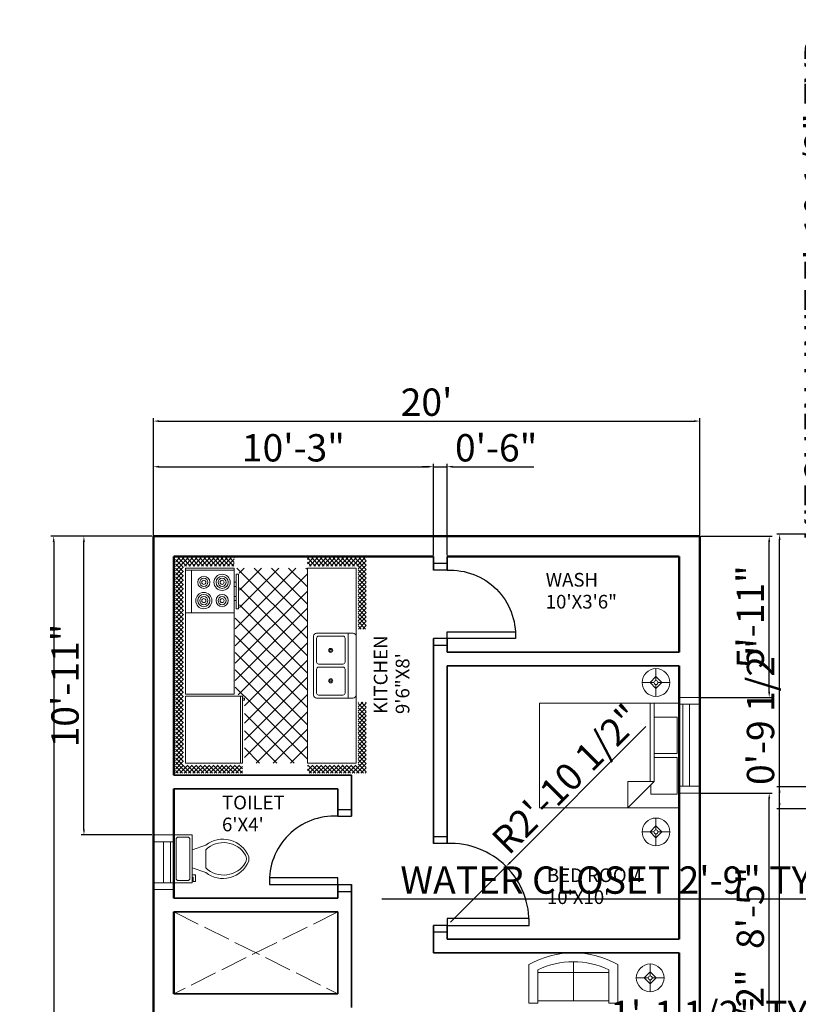
# Model space of a CAD drawing. Units: inches. Extents: x 2296 to 3335, y 495 to 1294.
# Tile 3 of 7: x 2296 to 2638, y 862 to 1294. Entities that reach past the tile are written whole.
import ezdxf

# ---------------------------------------------------------------- set-up
doc = ezdxf.new("R2010")
doc.units = ezdxf.units.IN
doc.linetypes.add('ACAD_ISO02W100', pattern=[15, 12, -3])
for name, color, linetype, lineweight in [('A-ANNO-DIMS', 2, 'Continuous', 18), ('A-AREA-IDEN', 7, 'Continuous', 18), ('A-FLOR-FIXT', 8, 'Continuous', 18), ('A-FLOR-OPEN', 7, 'ACAD_ISO02W100', 18), ('DOORS', 1, 'Continuous', 25), ('E-LITE', 2, 'Continuous', 18), ('FURNITURE', 2, 'Continuous', 18), ('INNER WALL', 6, 'Continuous', 35), ('OUTER WALL', 5, 'Continuous', 50), ('P-FIXT', 4, 'Continuous', 18), ('VENTILATOR', 4, 'Continuous', 18), ('WINDOWS', 3, 'Continuous', 18)]:
    doc.layers.add(name, color=color, linetype=linetype, lineweight=lineweight)
doc.styles.get("Standard").update_dxf_attribs({"font": 'arial.ttf'})
doc.dimstyles.new('ISO-25', dxfattribs={"dimtxt": 12, "dimasz": 2.5, "dimexe": 1.25, "dimexo": 0.625, "dimtad": 1, "dimdec": 1, "dimlunit": 3, "dimtxsty": 'Standard', "dimcen": 2.5, "dimadec": 0, "dimazin": 0, "dimtfac": 1, "dimtdec": 1, "dimtmove": 0, "dimatfit": 3, "dimfxl": 1, "dimarcsym": 0})

# ---------------------------------------------------------------- blocks, each defined once
blk = doc.blocks.new('Sofa - Roundback Loveseat 5 ft.')
for p, q in [((0, -32.44198), (0, -5.99998)), ((-24, -33.99998), (-24, -11.46958)), ((24.00004, -33.99998), (24.00004, -11.46958)), ((-23.9998, -13.38178), (23.99986, -13.38178)), ((-24, -32.44198), (24.00004, -32.44198))]:
    blk.add_line(p, q)
for points in [[(-24, -33.99998), (-30, -33.99998), (-30, -7.99998)], [(30.00004, -7.99998), (30.00004, -33.99998), (24.00004, -33.99998)]]:
    blk.add_lwpolyline(points)
for centre, radius, start, end in [((0, -60.24998), 60.24998, 60.13715, 119.8628), ((0, -61.38438), 55.38444, 64.32083, 115.6792)]:
    blk.add_arc(centre, radius, start, end)
blk = doc.blocks.new('Bed - Queen')
for p, q in [((0, -80.00003), (0, 0)), ((0, 0), (59.99999, 0)), ((59.99999, 0), (59.99999, -80.00003)), ((7.99999, -1.2), (28.79998, -1.2)), ((7.99999, -14.4), (7.99999, -1.2)), ((28.79998, -1.2), (28.79998, -14.4)), ((31.19999, -1.2), (51.99999, -1.2)), ((31.19999, -14.4), (31.19999, -1.2)), ((51.99999, -1.2), (51.99999, -16.4)), ((0, -14.4), (44.8, -14.4)), ((44.8, -16.8), (0, -16.8)), ((59.99999, -29.6), (44.8, -14.4)), ((44.8, -14.4), (44.8, -29.6)), ((51.99999, -16.4), (46.79936, -16.4)), ((44.8, -29.6), (59.99999, -29.6)), ((59.99999, -80.00003), (0, -80.00003))]:
    blk.add_line(p, q)
blk = doc.blocks.new('Kitchen Layout - 7 x 8 ft')
for p, q in [((-5, 81.32), (2.68, 89)), ((-5, 83.44), (0.56, 89)), ((-5, 85.56), (-1.56, 89)), ((-5, 87.68), (-3.68, 89)), ((-1, 84.97), (-5, 88.97)), ((1.09, 85), (-2.91, 89)), ((3.21, 85), (-0.79, 89)), ((0.81, 85), (4.81, 89)), ((5.34, 85), (1.34, 89)), ((2.93, 85), (6.93, 89)), ((7.46, 85), (3.46, 89)), ((5.05, 85), (9.05, 89)), ((9.58, 85), (5.58, 89)), ((7.17, 85), (11.17, 89)), ((11.7, 85), (7.7, 89)), ((9.29, 85), (13.29, 89)), ((13.82, 85), (9.82, 89)), ((11.41, 85), (15.41, 89)), ((15.94, 85), (11.94, 89)), ((13.53, 85), (17.53, 89)), ((18.06, 85), (14.06, 89)), ((15.65, 85), (19.65, 89)), ((20.18, 85), (16.18, 89)), ((17.78, 85), (21.78, 89)), ((22.31, 85), (18.31, 89)), ((19.9, 85), (23.9, 89)), ((24.43, 85), (20.43, 89)), ((22.02, 85), (26.02, 89)), ((26.55, 85), (22.55, 89)), ((24.14, 85), (28.14, 89)), ((28.67, 85), (24.67, 89)), ((26.26, 85), (30.26, 89)), ((30.79, 85), (26.79, 89)), ((28.38, 85), (32.38, 89)), ((32.91, 85), (28.91, 89)), ((30.5, 85), (34.5, 89)), ((35.03, 85), (31.03, 89)), ((32.63, 85), (36.63, 89)), ((37.16, 85), (33.16, 89)), ((34.75, 85), (38.75, 89)), ((39.28, 85), (35.28, 89)), ((36.87, 85), (40.87, 89)), ((41.4, 85), (37.4, 89)), ((38.99, 85), (42.99, 89)), ((43.52, 85), (39.52, 89)), ((41.11, 85), (45.11, 89)), ((45.64, 85), (41.64, 89)), ((43.23, 85), (47.23, 89)), ((47.76, 85), (43.76, 89)), ((45.35, 85), (49.35, 89)), ((49.88, 85), (45.88, 89)), ((47.47, 85), (51.47, 89)), ((52, 85), (48, 89)), ((49.6, 85), (53.6, 89)), ((54.13, 85), (50.13, 89)), ((51.72, 85), (55.72, 89)), ((56.25, 85), (52.25, 89)), ((53.84, 85), (57.84, 89)), ((58.37, 85), (54.37, 89)), ((55.96, 85), (59.96, 89)), ((60.49, 85), (56.49, 89)), ((58.08, 85), (62.08, 89)), ((62.61, 85), (58.61, 89)), ((60.2, 85), (64.2, 89)), ((64.73, 85), (60.73, 89)), ((62.32, 85), (66.32, 89)), ((66.85, 85), (62.85, 89)), ((64.45, 85), (68.45, 89)), ((68.97, 85), (64.97, 89)), ((66.57, 85), (70.57, 89)), ((71.1, 85), (67.1, 89)), ((68.69, 85), (72.69, 89)), ((73.22, 85), (69.22, 89)), ((70.81, 85), (74.81, 89)), ((75.34, 85), (71.34, 89)), ((72.93, 85), (76.93, 89)), ((77.46, 85), (73.46, 89)), ((75.05, 85), (79.05, 89)), ((79.58, 85), (75.58, 89)), ((77.17, 85), (81.17, 89)), ((81.7, 85), (77.7, 89)), ((79.29, 85), (83.29, 89)), ((83.82, 85), (79.82, 89)), ((81.42, 85), (85.42, 89)), ((85.95, 85), (81.95, 89)), ((83.54, 85), (87.54, 89)), ((88.07, 85), (84.07, 89)), ((85.66, 85), (89.66, 89)), ((90.19, 85), (86.19, 89)), ((87.78, 85), (91.78, 89)), ((92.31, 85), (88.31, 89)), ((89.9, 85), (93.9, 89)), ((94.43, 85), (90.43, 89)), ((92.02, 85), (96.02, 89)), ((96.55, 85), (92.55, 89)), ((94.14, 85), (98.14, 89)), ((101, 82.67), (94.67, 89)), ((96.27, 85), (100.27, 89)), ((101, 84.79), (96.79, 89)), ((97, 83.61), (101, 87.61)), ((101, 86.92), (98.92, 89)), ((-1, 82.85), (-5, 86.85)), ((-1, 80.73), (-5, 84.73)), ((-5, 79.19), (-1, 83.19)), ((-1, 78.61), (-5, 82.61)), ((34, 84), (96, 84)), ((34, 60), (34, 84)), ((96, 84), (96, 60)), ((97, 81.49), (101, 85.49)), ((101, 80.55), (97, 84.55)), ((97, 79.37), (101, 83.37)), ((101, 78.43), (97, 82.43)), ((-5, 77.07), (-1, 81.07)), ((-1, 76.49), (-5, 80.49)), ((-5, 74.95), (-1, 78.95)), ((-1, 74.36), (-5, 78.36)), ((74, 81), (95, 81)), ((97, 77.25), (101, 81.25)), ((101, 76.31), (97, 80.31)), ((97, 75.13), (101, 79.13)), ((101, 74.19), (97, 78.19)), ((-5, 72.83), (-1, 76.83)), ((-1, 72.24), (-5, 76.24)), ((-5, 70.71), (-1, 74.71)), ((-1, 70.12), (-5, 74.12)), ((97, 73.01), (101, 77.01)), ((101, 72.07), (97, 76.07)), ((97, 70.89), (101, 74.89)), ((101, 69.95), (97, 73.95)), ((97, 68.76), (101, 72.76)), ((-5, 68.59), (-1, 72.59)), ((-1, 68), (-5, 72)), ((-5, 66.47), (-1, 70.47)), ((-1, 65.88), (-5, 69.88)), ((-5, 64.35), (-1, 68.35)), ((101, 67.82), (97, 71.82)), ((97, 66.64), (101, 70.64)), ((101, 65.7), (97, 69.7)), ((97, 64.52), (101, 68.52)), ((-1, 63.76), (-5, 67.76)), ((-5, 62.22), (-1, 66.22)), ((-1, 61.64), (-5, 65.64)), ((-5, 60.1), (-1, 64.1)), ((-1, 59.52), (-5, 63.52)), ((101, 63.58), (97, 67.58)), ((97, 62.4), (101, 66.4)), ((101, 61.46), (97, 65.46)), ((97, 60.28), (101, 64.28)), ((100.34, 60), (97, 63.34)), ((-5, 57.98), (-1, 61.98)), ((-1, 57.39), (-5, 61.39)), ((-1.73, 56), (-5, 59.27)), ((-4.86, 56), (-1, 59.86)), ((10.4, 24), (45.9, 59.5)), ((18.88, 24), (54.38, 59.5)), ((27.37, 24), (62.87, 59.5)), ((33.03, 55.11), (37.41, 59.5)), ((96, 60), (34, 60)), ((35.85, 24), (71.35, 59.5)), ((76.2, 24), (40.7, 59.5)), ((84.68, 24), (49.18, 59.5)), ((93.17, 24), (57.67, 59.5)), ((61.31, 24), (96, 58.69)), ((96, 29.65), (66.15, 59.5)), ((80, 60), (80, 59)), ((82, 59), (82, 60)), ((87, 59), (87, 60)), ((89, 60), (89, 59)), ((98.22, 60), (97, 61.22)), ((98.84, 60), (101, 62.16)), ((100.96, 60), (101, 60.04)), ((-3.85, 56), (-5, 57.15)), ((-2.74, 56), (-1, 57.74)), ((0, 57), (33, 57)), ((0, 30.57), (24.43, 55)), ((0, 39.06), (15.94, 55)), ((0, 47.54), (7.46, 55)), ((1.91, 24), (32.91, 55)), ((33.77, 24), (2.77, 55)), ((42.26, 24), (11.26, 55)), ((50.74, 24), (19.74, 55)), ((59.23, 24), (28.23, 55)), ((31, 55), (31, 56)), ((32, 55), (31, 55)), ((32, 56), (32, 55)), ((67.71, 24), (33.68, 58.04)), ((44.34, 24), (77.84, 57.5)), ((52.82, 24), (86.32, 57.5)), ((96, 38.14), (76.64, 57.5)), ((96, 46.63), (85.13, 57.5)), ((96, 55.11), (93.57, 57.54)), ((25.29, 24), (0, 49.29)), ((69.79, 24), (96, 50.21)), ((16.8, 24), (0, 40.8)), ((78.28, 24), (96, 41.72)), ((8.32, 24), (0, 32.32)), ((86.76, 24), (96, 33.24)), ((95.25, 24), (96, 24.75)), ((-5, 21.92), (-2.92, 24)), ((-5, 19.8), (-1, 23.8)), ((-1, 19.21), (-5, 23.21)), ((-5, 17.68), (-1, 21.68)), ((-1, 17.09), (-5, 21.09)), ((-5, 15.55), (-1, 19.55)), ((-1, 21.33), (-3.67, 24)), ((-1, 23.45), (-1.55, 24)), ((0, 24), (96, 24)), ((0, 0), (0, 24)), ((96, 24), (96, 0)), ((97, 22.1), (98.9, 24)), ((97, 19.97), (101, 23.97)), ((101, 19.03), (97, 23.03)), ((97, 17.85), (101, 21.85)), ((101, 16.91), (97, 20.91)), ((97, 15.73), (101, 19.73)), ((101, 21.16), (98.16, 24)), ((101, 23.28), (100.28, 24)), ((-1, 14.97), (-5, 18.97)), ((-5, 13.43), (-1, 17.43)), ((-1, 12.85), (-5, 16.85)), ((-5, 11.31), (-1, 15.31)), ((-1, 10.73), (-5, 14.73)), ((47.25, 6.5), (47.25, 18.5)), ((48.75, 18.5), (48.75, 6.5)), ((101, 14.79), (97, 18.79)), ((97, 13.61), (101, 17.61)), ((101, 12.67), (97, 16.67)), ((97, 11.49), (101, 15.49)), ((101, 10.55), (97, 14.55)), ((-5, 9.19), (-1, 13.19)), ((-1, 8.6), (-5, 12.6)), ((-5, 7.07), (-1, 11.07)), ((-1, 6.48), (-5, 10.48)), ((97, 9.37), (101, 13.37)), ((101, 8.43), (97, 12.43)), ((97, 7.25), (101, 11.25)), ((101, 6.31), (97, 10.31)), ((-5, 4.95), (-1, 8.95)), ((-1, 4.36), (-5, 8.36)), ((-5, 2.83), (-1, 6.83)), ((-1, 2.24), (-5, 6.24)), ((97, 5.12), (101, 9.12)), ((101, 4.18), (97, 8.18)), ((97, 3), (101, 7)), ((101, 2.06), (97, 6.06)), ((97, 0.88), (101, 4.88)), ((-5, 0.71), (-1, 4.71)), ((-1, 0.12), (-5, 4.12)), ((-5, -1.42), (-1, 2.58)), ((2, -5), (-5, 2)), ((-5, -3.54), (-1, 0.46)), ((96, 0), (0, 0)), ((64, 4), (32, 4)), ((93.24, -5), (101, 2.76)), ((95.36, -5), (101, 0.64)), ((101, -0.06), (97, 3.94)), ((101, -2.18), (97, 1.82)), ((-0.12, -5), (-5, -0.12)), ((-2.25, -5), (-5, -2.25)), ((-4.37, -5), (-5, -4.37)), ((-4.34, -5), (-0.34, -1)), ((-2.22, -5), (1.78, -1)), ((-0.1, -5), (3.9, -1)), ((4.12, -5), (0.12, -1)), ((2.02, -5), (6.02, -1)), ((6.24, -5), (2.24, -1)), ((4.14, -5), (8.14, -1)), ((8.36, -5), (4.36, -1)), ((6.27, -5), (10.27, -1)), ((10.48, -5), (6.48, -1)), ((8.39, -5), (12.39, -1)), ((12.6, -5), (8.6, -1)), ((10.51, -5), (14.51, -1)), ((14.73, -5), (10.73, -1)), ((12.63, -5), (16.63, -1)), ((16.85, -5), (12.85, -1)), ((14.75, -5), (18.75, -1)), ((18.97, -5), (14.97, -1)), ((16.87, -5), (20.87, -1)), ((21.09, -5), (17.09, -1)), ((18.99, -5), (22.99, -1)), ((23.21, -5), (19.21, -1)), ((21.11, -5), (25.11, -1)), ((25.33, -5), (21.33, -1)), ((23.24, -5), (27.24, -1)), ((27.45, -5), (23.45, -1)), ((25.36, -5), (29.36, -1)), ((29.57, -5), (25.57, -1)), ((27.48, -5), (30, -2.48)), ((30, -3.3), (27.7, -1)), ((29.6, -5), (30, -4.6)), ((30, -1.18), (29.82, -1)), ((66, -2.54), (67.54, -1)), ((66, -4.66), (69.66, -1)), ((69.88, -5), (66, -1.12)), ((67.76, -5), (66, -3.24)), ((67.78, -5), (71.78, -1)), ((72, -5), (68, -1)), ((69.9, -5), (73.9, -1)), ((74.12, -5), (70.12, -1)), ((72.03, -5), (76.03, -1)), ((76.24, -5), (72.24, -1)), ((74.15, -5), (78.15, -1)), ((78.36, -5), (74.36, -1)), ((76.27, -5), (80.27, -1)), ((80.49, -5), (76.49, -1)), ((78.39, -5), (82.39, -1)), ((82.61, -5), (78.61, -1)), ((80.51, -5), (84.51, -1)), ((84.73, -5), (80.73, -1)), ((82.63, -5), (86.63, -1)), ((86.85, -5), (82.85, -1)), ((84.75, -5), (88.75, -1)), ((88.97, -5), (84.97, -1)), ((86.88, -5), (90.88, -1)), ((91.09, -5), (87.09, -1)), ((89, -5), (93, -1)), ((93.21, -5), (89.21, -1)), ((91.12, -5), (95.12, -1)), ((95.34, -5), (91.34, -1)), ((97.46, -5), (93.46, -1)), ((99.58, -5), (95.58, -1)), ((101, -4.3), (97, -0.3)), ((97.48, -5), (101, -1.48)), ((99.6, -5), (101, -3.6))]:
    blk.add_line(p, q)
for points in [[(0, 56), (0, 84), (33, 84), (33, 56)], [(74, 60), (74, 84), (95, 84), (95, 60)], [(76, 58), (76, 59), (93, 59), (93, 58)]]:
    blk.add_lwpolyline(points, close=True)
for points in [[(32, 1.5), (32, 19.5)], [(33.5, 21), (62.5, 21)], [(34.5, 19.5), (46.25, 19.5)], [(49.75, 19.5), (61.5, 19.5)], [(64, 19.5), (64, 1.5)], [(33.5, 6.5), (33.5, 18.5)], [(62.5, 18.5), (62.5, 6.5)], [(46.25, 5.5), (34.5, 5.5)], [(61.5, 5.5), (49.75, 5.5)], [(62.5, 0), (33.5, 0)]]:
    blk.add_lwpolyline(points)
for centre, radius in [((80, 75), 4), ((80, 75), 3), ((89, 75), 3), ((80, 75), 2), ((80, 75), 1), ((89, 75), 2), ((89, 75), 1), ((80, 66), 3), ((80, 66), 2), ((89, 66), 4), ((89, 66), 3), ((89, 66), 2), ((80, 66), 1), ((89, 66), 1), ((40.5, 12.5), 1), ((40.5, 12.5), 0.5), ((55.5, 12.5), 1), ((55.5, 12.5), 0.5)]:
    blk.add_circle(centre, radius)
for centre, radius, start, end in [((33.5, 19.5), 1.5, 90, 180), ((34.5, 18.5), 1, 90, 180), ((46.25, 18.5), 1, 0, 90), ((49.75, 18.5), 1, 90, 180), ((61.5, 18.5), 1, 0, 90), ((62.5, 19.5), 1.5, 0, 90), ((34.5, 6.5), 1, 180, 270), ((46.25, 6.5), 1, 270, 0), ((49.75, 6.5), 1, 180, 270), ((61.5, 6.5), 1, 270, 0), ((33.5, 1.5), 1.5, 180, 270), ((62.5, 1.5), 1.5, 270, 0)]:
    blk.add_arc(centre, radius, start, end)
blk = doc.blocks.new('Lamp - Table')
for p, q in [((0, 7), (0, 1)), ((-1, 0), (-7, 0)), ((0, 3), (-3, 0)), ((-3, 0), (0, -3)), ((3, 0), (0, 3)), ((0, -3), (3, 0)), ((1, 0), (7, 0)), ((0, -1), (0, -7))]:
    blk.add_line(p, q)
for radius in [7, 1]:
    blk.add_circle((0, 0), radius)
blk = doc.blocks.new('Toilet - top')
for p, q in [((9.5, -6), (9.5, -2)), ((-10, -8.5), (-8, -8.5)), ((-10, -9.5), (-10, -8.5)), ((-8, -8.5), (-8, -8)), ((-7, -8), (-7, -9.5)), ((-4, -8), (-6, -14)), ((4, -8), (6, -14)), ((-7, -9.5), (-10, -9.5)), ((4, -14), (-4, -14))]:
    blk.add_line(p, q)
blk.add_lwpolyline([(10.5, -8), (10.5, 0), (-10.5, 0), (-10.5, -8)], close=True)
for points in [[(-9.5, -2), (-9.5, -6)], [(8.5, -1), (-8.5, -1)], [(-8.5, -7), (8.5, -7)]]:
    blk.add_lwpolyline(points)
for centre, radius, start, end in [((-8.62, -1.88), 0.884, 81.8699, 188.1301), ((8.62, -1.88), 0.884, 351.8699, 98.1301), ((-8.62, -6.12), 0.884, 171.8699, 278.1301), ((8.62, -6.12), 0.884, 261.8699, 8.1301), ((3.52, -21.58), 12.17, 141.4691, 247.9714), ((4.2, -21.82), 11.33, 136.3677, 238.9468), ((-3.52, -21.58), 12.17, 292.0284, 38.5307), ((-4.2, -21.82), 11.33, 301.053, 43.6321), ((0, -27.88), 4, 245.7318, 294.2682), ((0, -29), 4, 254.8605, 285.1395)]:
    blk.add_arc(centre, radius, start, end)
blk = doc.blocks.new('*D16')
at = {"layer": 'A-ANNO-DIMS', "color": 0, "lineweight": -2, "transparency": 16777216}
for p, q in [((2355.08, 1067.77), (2355.08, 1118.94)), ((2357.58, 1117.69), (2592.58, 1117.69)), ((2595.08, 1067.77), (2595.08, 1118.94))]:
    blk.add_line(p, q, dxfattribs=at)
at = {"layer": 'A-ANNO-DIMS', "color": 0, "transparency": 16777216}
for points in [[(2357.58, 1118.1), (2357.58, 1117.27), (2355.08, 1117.69)], [(2592.58, 1118.1), (2592.58, 1117.27), (2595.08, 1117.69)]]:
    blk.add_solid(points, dxfattribs=at)
at = {"layer": 'Defpoints', "color": 0, "transparency": 16777216}
for p in [(2595.08, 1117.69), (2355.08, 1067.15), (2595.08, 1067.15)]:
    blk.add_point(p, dxfattribs=at)
at = {"layer": 'A-ANNO-DIMS', "color": 0, "transparency": 16777216, "insert": (2475.08, 1124.44), "char_height": 12, "attachment_point": 5}
blk.add_mtext("20'", dxfattribs=at)
blk = doc.blocks.new('*D17')
at = {"layer": 'A-ANNO-DIMS', "color": 0, "lineweight": -2, "transparency": 16777216}
for p, q in [((2354.45, 1067.15), (2310.04, 1067.15)), ((2311.29, 1064.65), (2311.29, 589.65)), ((2354.45, 587.15), (2310.04, 587.15))]:
    blk.add_line(p, q, dxfattribs=at)
at = {"layer": 'A-ANNO-DIMS', "color": 0, "transparency": 16777216}
for points in [[(2310.87, 1064.65), (2311.7, 1064.65), (2311.29, 1067.15)], [(2310.87, 589.65), (2311.7, 589.65), (2311.29, 587.15)]]:
    blk.add_solid(points, dxfattribs=at)
at = {"layer": 'Defpoints', "color": 0, "transparency": 16777216}
for p in [(2355.08, 1067.15), (2311.29, 587.15), (2355.08, 587.15)]:
    blk.add_point(p, dxfattribs=at)
at = {"layer": 'A-ANNO-DIMS', "color": 0, "transparency": 16777216, "insert": (2304.54, 827.15), "char_height": 12, "attachment_point": 5, "rotation": 90}
blk.add_mtext("40'", dxfattribs=at)
blk = doc.blocks.new('DOOR-SINGLE-30IN')
for p, q in [((-3, 0), (-3, -6)), ((0, 0), (0, -6)), ((30, 0), (30, -6)), ((33, 0), (33, -6))]:
    blk.add_line(p, q)
blk.add_lwpolyline([(0, 0), (3, 0), (3, 30), (0, 30)], close=True)
blk.add_arc((1.5, 1.5), 28.54, 356.9872, 93.0128)
blk = doc.blocks.new('DOOR-SINGLE-36IN')
for p, q in [((0, 39), (-6, 39)), ((0, 36), (-6, 36)), ((0, 0), (-6, 0)), ((0, -3), (-6, -3))]:
    blk.add_line(p, q)
blk.add_lwpolyline([(0, 0), (36, 0), (36, 3), (0, 3)], close=True)
blk.add_arc((1.5, 1.5), 34.53, 357.5104, 92.4896)
blk = doc.blocks.new('WIN-36IN')
for p, q in [((0, 42), (9, 42)), ((0, 39), (9, 39)), ((1.5, 3), (1.5, 39)), ((4.5, 3), (4.5, 39)), ((9, 3), (0, 3)), ((9, 0), (0, 0))]:
    blk.add_line(p, q)
blk = doc.blocks.new('VENT-18IN')
for p, q in [((0, 24), (9, 24)), ((0, 21), (9, 21)), ((4.5, 21), (4.5, 3)), ((7.5, 21), (7.5, 3)), ((9, 3), (0, 3)), ((9, 0), (0, 0))]:
    blk.add_line(p, q)
blk = doc.blocks.new('FLOOR-OPENING-72X36')
for p, q in [((0, 36), (72, 0)), ((72, 36), (0, 0))]:
    blk.add_line(p, q)
blk = doc.blocks.new('*D25')
at = {"layer": 'A-ANNO-DIMS', "color": 0, "lineweight": -2, "transparency": 16777216}
for p, q in [((2655.47, 1058.33), (2655.47, 1293.98)), ((2669.03, 1058.33), (2654.22, 1058.33)), ((2655.47, 966.25), (2655.47, 1055.83)), ((2669.03, 963.75), (2654.22, 963.75))]:
    blk.add_line(p, q, dxfattribs=at)
at = {"layer": 'A-ANNO-DIMS', "color": 0, "transparency": 16777216}
for points in [[(2655.05, 1055.83), (2655.89, 1055.83), (2655.47, 1058.33)], [(2655.05, 966.25), (2655.89, 966.25), (2655.47, 963.75)]]:
    blk.add_solid(points, dxfattribs=at)
at = {"layer": 'Defpoints', "color": 0, "transparency": 16777216}
for p in [(2655.47, 1058.33), (2669.66, 1058.33), (2669.66, 963.75)]:
    blk.add_point(p, dxfattribs=at)
at = {"layer": 'A-ANNO-DIMS', "color": 0, "transparency": 16777216, "insert": (2648.64, 1177.41), "char_height": 12, "attachment_point": 5, "rotation": 90}
blk.add_mtext('KITCHEN UNIT 7\'-10 1/2" TYP.', dxfattribs=at)
blk = doc.blocks.new('*D31')
at = {"layer": 'A-ANNO-DIMS', "color": 0, "lineweight": -2, "transparency": 16777216}
for p, q in [((2669.71, 912.04), (2669.71, 906.46)), ((2702.75, 912.04), (2702.75, 906.46)), ((2669.71, 907.71), (2455.4, 907.71)), ((2700.25, 907.71), (2672.21, 907.71))]:
    blk.add_line(p, q, dxfattribs=at)
at = {"layer": 'A-ANNO-DIMS', "color": 0, "transparency": 16777216}
for points in [[(2672.21, 908.12), (2672.21, 907.29), (2669.71, 907.71)], [(2700.25, 908.12), (2700.25, 907.29), (2702.75, 907.71)]]:
    blk.add_solid(points, dxfattribs=at)
at = {"layer": 'Defpoints', "color": 0, "transparency": 16777216}
for p in [(2669.71, 912.66), (2702.75, 912.66), (2669.71, 907.71)]:
    blk.add_point(p, dxfattribs=at)
at = {"layer": 'A-ANNO-DIMS', "color": 0, "transparency": 16777216, "insert": (2561.3, 914.54), "char_height": 12, "attachment_point": 5}
blk.add_mtext('WATER CLOSET 2\'-9" TYP.', dxfattribs=at)
blk = doc.blocks.new('*D46')
at = {"layer": 'A-ANNO-DIMS', "color": 0, "lineweight": -2, "transparency": 16777216}
for p, q in [((2539.71, 845.21), (2539.71, 849.93)), ((2542.21, 848.68), (2550.88, 848.68)), ((2553.38, 845.21), (2553.38, 849.93)), ((2553.38, 848.68), (2657.11, 848.68))]:
    blk.add_line(p, q, dxfattribs=at)
at = {"layer": 'A-ANNO-DIMS', "color": 0, "transparency": 16777216}
for points in [[(2542.21, 849.1), (2542.21, 848.27), (2539.71, 848.68)], [(2550.88, 849.1), (2550.88, 848.27), (2553.38, 848.68)]]:
    blk.add_solid(points, dxfattribs=at)
at = {"layer": 'Defpoints', "color": 0, "transparency": 16777216}
for p in [(2553.38, 848.68), (2539.71, 844.58), (2553.38, 844.58)]:
    blk.add_point(p, dxfattribs=at)
at = {"layer": 'A-ANNO-DIMS', "color": 0, "transparency": 16777216, "insert": (2606.5, 855.51), "char_height": 12, "attachment_point": 5}
blk.add_mtext('1\'-1 1/2" TYP.', dxfattribs=at)
blk = doc.blocks.new('*D52')
at = {"layer": 'A-ANNO-DIMS', "color": 0, "lineweight": -2, "transparency": 16777216}
for p, q in [((2660.03, 1068.02), (2628.91, 1068.02)), ((2630.16, 590.52), (2630.16, 1065.52)), ((2660.03, 588.02), (2628.91, 588.02))]:
    blk.add_line(p, q, dxfattribs=at)
at = {"layer": 'A-ANNO-DIMS', "color": 0, "transparency": 16777216}
for points in [[(2629.74, 1065.52), (2630.57, 1065.52), (2630.16, 1068.02)], [(2629.74, 590.52), (2630.57, 590.52), (2630.16, 588.02)]]:
    blk.add_solid(points, dxfattribs=at)
at = {"layer": 'Defpoints', "color": 0, "transparency": 16777216}
for p in [(2630.16, 1068.02), (2660.66, 1068.02), (2660.66, 588.02)]:
    blk.add_point(p, dxfattribs=at)
at = {"layer": 'A-ANNO-DIMS', "color": 0, "transparency": 16777216, "insert": (2623.41, 828.02), "char_height": 12, "attachment_point": 5, "rotation": 90}
blk.add_mtext('40\'-0"', dxfattribs=at)
blk = doc.blocks.new('*D55')
at = {"layer": 'A-ANNO-DIMS', "color": 0, "lineweight": -2, "transparency": 16777216}
for p, q in [((2595.7, 1067.15), (2626.83, 1067.15)), ((2625.58, 998.8), (2625.58, 1064.65)), ((2595.7, 996.3), (2626.83, 996.3))]:
    blk.add_line(p, q, dxfattribs=at)
at = {"layer": 'A-ANNO-DIMS', "color": 0, "transparency": 16777216}
for points in [[(2625.16, 1064.65), (2625.99, 1064.65), (2625.58, 1067.15)], [(2625.16, 998.8), (2625.99, 998.8), (2625.58, 996.3)]]:
    blk.add_solid(points, dxfattribs=at)
at = {"layer": 'Defpoints', "color": 0, "transparency": 16777216}
for p in [(2595.08, 1067.15), (2625.58, 1067.15), (2595.08, 996.3)]:
    blk.add_point(p, dxfattribs=at)
at = {"layer": 'A-ANNO-DIMS', "color": 0, "transparency": 16777216, "insert": (2618.83, 1031.72), "char_height": 12, "attachment_point": 5, "rotation": 90}
blk.add_mtext('5\'-11"', dxfattribs=at)
blk = doc.blocks.new('*D56')
at = {"layer": 'A-ANNO-DIMS', "color": 0, "lineweight": -2, "transparency": 16777216}
for p, q in [((2595.7, 954.3), (2626.83, 954.3)), ((2625.58, 855.97), (2625.58, 951.8)), ((2595.7, 853.47), (2626.83, 853.47))]:
    blk.add_line(p, q, dxfattribs=at)
at = {"layer": 'A-ANNO-DIMS', "color": 0, "transparency": 16777216}
for points in [[(2625.16, 951.8), (2625.99, 951.8), (2625.58, 954.3)], [(2625.16, 855.97), (2625.99, 855.97), (2625.58, 853.47)]]:
    blk.add_solid(points, dxfattribs=at)
at = {"layer": 'Defpoints', "color": 0, "transparency": 16777216}
for p in [(2595.08, 954.3), (2625.58, 954.3), (2595.08, 853.47)]:
    blk.add_point(p, dxfattribs=at)
at = {"layer": 'A-ANNO-DIMS', "color": 0, "transparency": 16777216, "insert": (2618.83, 903.89), "char_height": 12, "attachment_point": 5, "rotation": 90}
blk.add_mtext('8\'-5"', dxfattribs=at)
blk = doc.blocks.new('*D57')
at = {"layer": 'A-ANNO-DIMS', "color": 0, "lineweight": -2, "transparency": 16777216}
for p, q in [((2625.58, 811.47), (2625.58, 875.57)), ((2595.7, 811.47), (2626.83, 811.47)), ((2625.58, 762.3), (2625.58, 808.97)), ((2595.7, 759.8), (2626.83, 759.8))]:
    blk.add_line(p, q, dxfattribs=at)
at = {"layer": 'A-ANNO-DIMS', "color": 0, "transparency": 16777216}
for points in [[(2625.16, 808.97), (2625.99, 808.97), (2625.58, 811.47)], [(2625.16, 762.3), (2625.99, 762.3), (2625.58, 759.8)]]:
    blk.add_solid(points, dxfattribs=at)
at = {"layer": 'Defpoints', "color": 0, "transparency": 16777216}
for p in [(2595.08, 811.47), (2625.58, 811.47), (2595.08, 759.8)]:
    blk.add_point(p, dxfattribs=at)
at = {"layer": 'A-ANNO-DIMS', "color": 0, "transparency": 16777216, "insert": (2618.74, 844.77), "char_height": 12, "attachment_point": 5, "rotation": 90}
blk.add_mtext('4\'-3 1/2"', dxfattribs=at)
blk = doc.blocks.new('*D58')
at = {"layer": 'A-ANNO-DIMS', "color": 0, "lineweight": -2, "transparency": 16777216}
for p, q in [((2354.45, 1067.15), (2323.33, 1067.15)), ((2324.58, 938.42), (2324.58, 1064.65)), ((2354.45, 935.92), (2323.33, 935.92))]:
    blk.add_line(p, q, dxfattribs=at)
at = {"layer": 'A-ANNO-DIMS', "color": 0, "transparency": 16777216}
for points in [[(2324.16, 1064.65), (2324.99, 1064.65), (2324.58, 1067.15)], [(2324.16, 938.42), (2324.99, 938.42), (2324.58, 935.92)]]:
    blk.add_solid(points, dxfattribs=at)
at = {"layer": 'Defpoints', "color": 0, "transparency": 16777216}
for p in [(2324.58, 1067.15), (2355.08, 1067.15), (2355.08, 935.92)]:
    blk.add_point(p, dxfattribs=at)
at = {"layer": 'A-ANNO-DIMS', "color": 0, "transparency": 16777216, "insert": (2317.83, 1001.53), "char_height": 12, "attachment_point": 5, "rotation": 90}
blk.add_mtext('10\'-11"', dxfattribs=at)
blk = doc.blocks.new('*D64')
at = {"layer": 'A-ANNO-DIMS', "color": 0, "lineweight": -2, "transparency": 16777216}
for p, q in [((2355.08, 1067.77), (2355.08, 1098.9)), ((2478.08, 1058.77), (2478.08, 1098.9)), ((2357.58, 1097.65), (2475.58, 1097.65))]:
    blk.add_line(p, q, dxfattribs=at)
at = {"layer": 'A-ANNO-DIMS', "color": 0, "transparency": 16777216}
for points in [[(2357.58, 1098.06), (2357.58, 1097.23), (2355.08, 1097.65)], [(2475.58, 1098.06), (2475.58, 1097.23), (2478.08, 1097.65)]]:
    blk.add_solid(points, dxfattribs=at)
at = {"layer": 'Defpoints', "color": 0, "transparency": 16777216}
for p in [(2478.08, 1097.65), (2355.08, 1067.15), (2478.08, 1058.15)]:
    blk.add_point(p, dxfattribs=at)
at = {"layer": 'A-ANNO-DIMS', "color": 0, "transparency": 16777216, "insert": (2416.58, 1104.4), "char_height": 12, "attachment_point": 5}
blk.add_mtext('10\'-3"', dxfattribs=at)
blk = doc.blocks.new('*D65')
at = {"layer": 'A-ANNO-DIMS', "color": 0, "lineweight": -2, "transparency": 16777216}
for p, q in [((2478.08, 1058.77), (2478.08, 1098.9)), ((2484.08, 1058.77), (2484.08, 1098.9)), ((2475.58, 1097.65), (2473.08, 1097.65)), ((2478.08, 1097.65), (2484.08, 1097.65)), ((2486.58, 1097.65), (2522.23, 1097.65))]:
    blk.add_line(p, q, dxfattribs=at)
at = {"layer": 'A-ANNO-DIMS', "color": 0, "transparency": 16777216}
for points in [[(2475.58, 1098.06), (2475.58, 1097.23), (2478.08, 1097.65)], [(2486.58, 1098.06), (2486.58, 1097.23), (2484.08, 1097.65)]]:
    blk.add_solid(points, dxfattribs=at)
at = {"layer": 'Defpoints', "color": 0, "transparency": 16777216}
for p in [(2484.08, 1097.65), (2478.08, 1058.15), (2484.08, 1058.15)]:
    blk.add_point(p, dxfattribs=at)
at = {"layer": 'A-ANNO-DIMS', "color": 0, "transparency": 16777216, "insert": (2505.65, 1104.4), "char_height": 12, "attachment_point": 5}
blk.add_mtext('0\'-6"', dxfattribs=at)
blk = doc.blocks.new('*D70')
at = {"layer": 'A-ANNO-DIMS', "color": 0, "lineweight": -2, "transparency": 16777216}
for p, q in [((2630.16, 957.02), (2630.16, 1020.63)), ((2669.03, 957.02), (2628.91, 957.02)), ((2630.16, 949.9), (2630.16, 954.52)), ((2669.03, 947.4), (2628.91, 947.4))]:
    blk.add_line(p, q, dxfattribs=at)
at = {"layer": 'A-ANNO-DIMS', "color": 0, "transparency": 16777216}
for points in [[(2629.74, 954.52), (2630.57, 954.52), (2630.16, 957.02)], [(2629.74, 949.9), (2630.57, 949.9), (2630.16, 947.4)]]:
    blk.add_solid(points, dxfattribs=at)
at = {"layer": 'Defpoints', "color": 0, "transparency": 16777216}
for p in [(2630.16, 957.02), (2669.66, 957.02), (2669.66, 947.4)]:
    blk.add_point(p, dxfattribs=at)
at = {"layer": 'A-ANNO-DIMS', "color": 0, "transparency": 16777216, "insert": (2623.33, 990.07), "char_height": 12, "attachment_point": 5, "rotation": 90}
blk.add_mtext('0\'-9 1/2"', dxfattribs=at)
blk = doc.blocks.new('*D79')
at = {"layer": 'A-ANNO-DIMS', "color": 0, "lineweight": -2, "transparency": 16777216}
for p, q in [((2571.46, 983.52), (2511.76, 923.83)), ((2485.58, 897.65), (2510, 922.06))]:
    blk.add_line(p, q, dxfattribs=at)
at = {"layer": 'A-ANNO-DIMS', "color": 0, "transparency": 16777216}
blk.add_solid([(2511.47, 924.13), (2512.06, 923.54), (2510, 922.06)], dxfattribs=at)
at = {"layer": 'Defpoints', "color": 0, "transparency": 16777216}
for p in [(2510, 922.06), (2485.58, 897.65)]:
    blk.add_point(p, dxfattribs=at)
at = {"layer": 'A-ANNO-DIMS', "color": 0, "transparency": 16777216, "insert": (2537.67, 959.39), "char_height": 12, "attachment_point": 5, "rotation": 45.0001}
blk.add_mtext('R2\'-10 1/2"', dxfattribs=at)

msp = doc.modelspace()

# ---------------------------------------------------------------- linework, layer by layer
at = {"layer": 'INNER WALL'}
for p, q in [((2478.08, 1058.15), (2478.08, 1052.15)), ((2484.08, 1058.15), (2484.08, 1052.15)), ((2478.08, 1022.15), (2478.08, 956.15)), ((2484.08, 1022.15), (2484.08, 1016.15)), ((2586.08, 1016.15), (2484.08, 1016.15)), ((2586.08, 1010.15), (2484.08, 1010.15)), ((2484.08, 1010.15), (2484.08, 932.15)), ((2442.08, 962.15), (2364.08, 962.15)), ((2442.08, 962.15), (2442.08, 944.15)), ((2436.08, 956.15), (2364.08, 956.15)), ((2436.08, 956.15), (2436.08, 944.15)), ((2478.08, 956.15), (2478.08, 932.15)), ((2436.08, 914.15), (2436.08, 908.15)), ((2442.08, 914.15), (2442.08, 860.15)), ((2436.08, 908.15), (2364.08, 908.15)), ((2436.08, 902.15), (2364.08, 902.15)), ((2436.08, 902.15), (2436.08, 866.15)), ((2478.08, 896.15), (2478.08, 884.15)), ((2484.08, 896.15), (2484.08, 890.15)), ((2586.08, 890.15), (2484.08, 890.15)), ((2586.08, 884.15), (2478.08, 884.15)), ((2436.08, 866.15), (2364.08, 866.15))]:
    msp.add_line(p, q, dxfattribs=at)
at = {"layer": 'OUTER WALL'}
for p, q in [((2364.08, 1058.15), (2364.08, 962.15)), ((2478.08, 1058.15), (2364.08, 1058.15)), ((2586.08, 1058.15), (2484.08, 1058.15)), ((2586.08, 1016.15), (2586.08, 1058.15)), ((2586.08, 890.15), (2586.08, 1010.15)), ((2364.08, 956.15), (2364.08, 908.15)), ((2364.08, 902.15), (2364.08, 866.15)), ((2586.08, 782.15), (2586.08, 884.15))]:
    msp.add_line(p, q, dxfattribs=at)
msp.add_lwpolyline([(2460.08, 587.15), (2595.08, 587.15), (2595.08, 1067.15), (2355.08, 1067.15), (2355.08, 587.15), (2364.08, 587.15)], dxfattribs=at)

# ---------------------------------------------------------------- block references
at = {"layer": 'A-FLOR-FIXT', "xscale": 0.8922679191465929, "yscale": 0.8922679191465929, "zscale": 0.8922679191465929, "rotation": 90.00000000002456}
msp.add_blockref('Kitchen Layout - 7 x 8 ft', (2444.16, 967.46), dxfattribs=at)
at = {"layer": 'A-FLOR-OPEN'}
msp.add_blockref('FLOOR-OPENING-72X36', (2364.08, 866.15), dxfattribs=at)
at = {"layer": 'DOORS', "extrusion": (0, 0, -1), "zscale": -1, "rotation": 89.99999999999824}
msp.add_blockref('DOOR-SINGLE-30IN', (-2484.08, 1022.15), dxfattribs=at)
at = {"layer": 'DOORS', "rotation": 89.99999999999808}
msp.add_blockref('DOOR-SINGLE-30IN', (2436.08, 914.15), dxfattribs=at)
at = {"layer": 'DOORS'}
msp.add_blockref('DOOR-SINGLE-36IN', (2484.08, 896.15), dxfattribs=at)
at = {"layer": 'E-LITE', "xscale": 0.8700180084150424, "yscale": 0.8700180084150424, "zscale": 0.8700180084150424}
for p in [(2575.85, 1002.86), (2575.85, 937.27), (2573.31, 873.15)]:
    msp.add_blockref('Lamp - Table', p, dxfattribs=at)
at = {"layer": 'FURNITURE', "xscale": 0.7674836837443932, "yscale": 0.7674836837443932, "zscale": 0.7674836837443932, "rotation": 270}
msp.add_blockref('Bed - Queen', (2586.14, 993.81), dxfattribs=at)
at = {"layer": 'FURNITURE', "xscale": 0.6498910467683475, "yscale": 0.6498910467683475, "zscale": 0.6498910467683475}
msp.add_blockref('Sofa - Roundback Loveseat 5 ft.', (2539.56, 884.15), dxfattribs=at)
at = {"layer": 'P-FIXT', "rotation": 90}
msp.add_blockref('Toilet - top', (2364.08, 925.42), dxfattribs=at)
at = {"layer": 'VENTILATOR'}
msp.add_blockref('VENT-18IN', (2355.08, 911.92), dxfattribs=at)
at = {"layer": 'WINDOWS'}
msp.add_blockref('WIN-36IN', (2586.08, 954.3), dxfattribs=at)

# ---------------------------------------------------------------- texts
at = {"layer": 'A-AREA-IDEN'}
for s, p in [('WASH', (2527.42, 1045)), ('10\'X3\'6"', (2527.42, 1035.36)), ('TOILET', (2385.22, 947.16)), ("6'X4'", (2385.22, 937.52)), ('BED ROOM', (2527.96, 915.22)), ("10'X10'", (2527.96, 905.58))]:
    msp.add_text(s, height=6, dxfattribs=at).set_placement(p)
for s, p in [('KITCHEN', (2457.89, 989.02)), ('9\'6"X8\'', (2467.53, 989.02))]:
    msp.add_text(s, height=6, rotation=90, dxfattribs=at).set_placement(p)

# ---------------------------------------------------------------- dimensions: what is measured, and where the dimension line sits
at = {"layer": 'A-ANNO-DIMS'}
for base, p1, p2, angle, text, picture, middle in [((2655.47, 1058.33), (2669.66, 963.75), (2669.66, 1058.33), 90, 'KITCHEN UNIT <> TYP.', '*D25', (2648.64, 1177.41)), ((2669.71, 907.71), (2702.75, 912.66), (2669.71, 912.66), 180, 'WATER CLOSET <> TYP.', '*D31', (2561.3, 914.54))]:
    dim = msp.add_linear_dim(base=base, p1=p1, p2=p2, angle=angle, text=text, dimstyle='ISO-25', override={"dimdec": 1, "dimlfac": 1, "dimrnd": 0, "dimzin": 1, "dimdsep": 46, "dimlunit": 4, "dimfrac": 2}, dxfattribs=at)
    dim.commit()
    dim.dimension.update_dxf_attribs({"geometry": picture, "text_midpoint": middle})
for base, p1, p2, override, picture, middle in [((2595.08, 1117.69), (2355.08, 1067.15), (2595.08, 1067.15), {"dimclrd": 0, "dimclre": 0, "dimclrt": 0}, '*D16', (2475.08, 1124.44)), ((2478.08, 1097.65), (2355.08, 1067.15), (2478.08, 1058.15), {"dimdec": 1, "dimlfac": 1, "dimrnd": 0, "dimzin": 1, "dimdsep": 46, "dimlunit": 4, "dimfrac": 2}, '*D64', (2416.58, 1104.4)), ((2484.08, 1097.65), (2478.08, 1058.15), (2484.08, 1058.15), {"dimdec": 1, "dimlfac": 1, "dimrnd": 0, "dimzin": 1, "dimdsep": 46, "dimlunit": 4, "dimfrac": 2}, '*D65', (2505.65, 1104.4))]:
    dim = msp.add_linear_dim(base=base, p1=p1, p2=p2, dimstyle='ISO-25', override=override, dxfattribs=at)
    dim.commit()
    dim.dimension.update_dxf_attribs({"geometry": picture, "text_midpoint": middle})
for base, p1, p2, override, picture, middle in [((2311.29, 587.15), (2355.08, 1067.15), (2355.08, 587.15), {"dimclrd": 0, "dimclre": 0, "dimclrt": 0}, '*D17', (2304.54, 827.15)), ((2324.58, 1067.15), (2355.08, 935.92), (2355.08, 1067.15), {"dimdec": 1, "dimlfac": 1, "dimrnd": 0, "dimzin": 1, "dimdsep": 46, "dimlunit": 4, "dimfrac": 2}, '*D58', (2317.83, 1001.53)), ((2625.5782, 1067.1452), (2595.0782, 996.3047), (2595.0782, 1067.1452), {"dimdec": 1, "dimlfac": 1, "dimrnd": 0, "dimzin": 1, "dimdsep": 46, "dimlunit": 4, "dimfrac": 2}, '*D55', (2618.8263, 1031.7249)), ((2630.16, 1068.02), (2660.66, 588.02), (2660.66, 1068.02), {"dimdec": 1, "dimlfac": 1, "dimrnd": 0, "dimzin": 1, "dimdsep": 46, "dimlunit": 4, "dimfrac": 2}, '*D52', (2623.41, 828.02)), ((2630.16, 957.02), (2669.66, 947.4), (2669.66, 957.02), {"dimdec": 1, "dimlfac": 1, "dimrnd": 0, "dimzin": 1, "dimdsep": 46, "dimlunit": 4, "dimfrac": 2}, '*D70', (2623.33, 990.07)), ((2625.58, 954.3), (2595.08, 853.47), (2595.08, 954.3), {"dimdec": 1, "dimlfac": 1, "dimrnd": 0, "dimzin": 1, "dimdsep": 46, "dimlunit": 4, "dimfrac": 2}, '*D56', (2618.83, 903.89)), ((2625.58, 811.47), (2595.08, 759.8), (2595.08, 811.47), {"dimdec": 1, "dimlfac": 1, "dimrnd": 0, "dimzin": 1, "dimdsep": 46, "dimlunit": 4, "dimfrac": 2}, '*D57', (2618.74, 844.77))]:
    dim = msp.add_linear_dim(base=base, p1=p1, p2=p2, angle=90, dimstyle='ISO-25', override=override, dxfattribs=at)
    dim.commit()
    dim.dimension.update_dxf_attribs({"geometry": picture, "text_midpoint": middle})
dim = msp.add_radius_dim(center=(2485.58, 897.65), mpoint=(2510, 922.06), dimstyle='ISO-25', override={"dimdec": 1, "dimlfac": 1, "dimrnd": 0, "dimzin": 1, "dimdsep": 46, "dimlunit": 4, "dimfrac": 2}, dxfattribs=at)
dim.commit()
dim.dimension.update_dxf_attribs({"geometry": '*D79', "text_midpoint": (2537.67, 959.39)})
dim = msp.add_linear_dim(base=(2553.38, 848.68), p1=(2539.71, 844.58), p2=(2553.38, 844.58), text='<> TYP.', dimstyle='ISO-25', override={"dimdec": 1, "dimlfac": 1, "dimrnd": 0, "dimzin": 1, "dimdsep": 46, "dimlunit": 4, "dimfrac": 2}, dxfattribs=at)
dim.commit()
dim.dimension.update_dxf_attribs({"geometry": '*D46', "text_midpoint": (2606.5, 855.51)})

doc.saveas('drawing.dxf')
